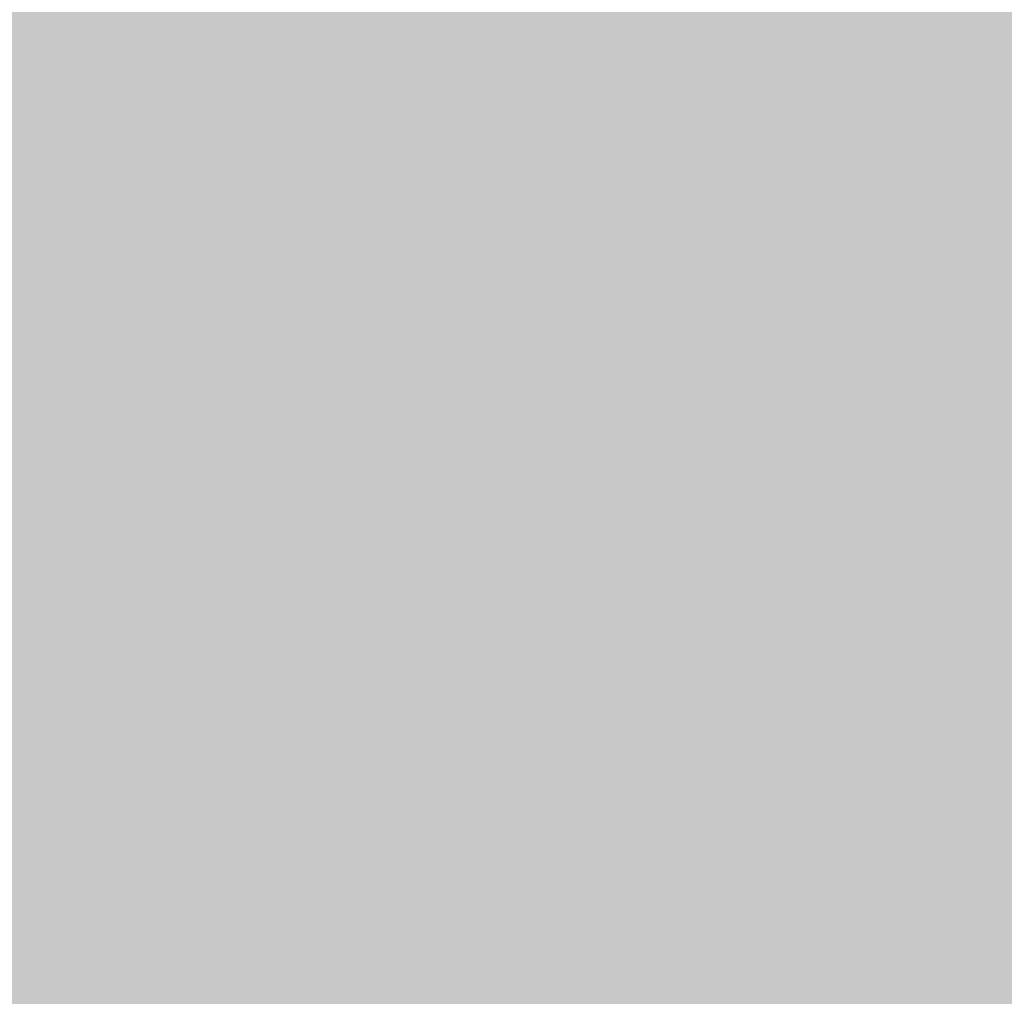
# Model space of a CAD drawing. Units: inches. Extents: x 2083 to 3317, y 1141 to 2115.
# Tile 160 of 256: x 3126.955939 to 3126.958245, y 1263.263648 to 1263.265937. Entities that reach past the tile are written whole.
import ezdxf

# ---------------------------------------------------------------- set-up
doc = ezdxf.new("R2010")
doc.units = ezdxf.units.IN
doc.layers.add('A-WALL-PATT', color=251, linetype='Continuous', lineweight=13, true_color=0x636466)

msp = doc.modelspace()

# ---------------------------------------------------------------- hatches: boundary and pattern name
at = {"layer": 'A-WALL-PATT'}
h = msp.add_hatch(color=256, dxfattribs=at)
h.dxf.hatch_style = 1
h.paths.add_polyline_path([(3126.9597832, 2020.7613601), (2748.9597832, 2020.7613601), (2604.9597832, 2020.7613601), (2226.9597832, 2020.7613601), (2226.9597832, 1702.7613601), (2466.9597832, 1702.7613601), (2466.9597832, 1582.7613601), (2418.9597832, 1582.7613601), (2418.9597832, 1477.7613601), (2226.9597832, 1477.7613601), (2226.9597832, 1263.2613601), (2544.9597832, 1263.2613601), (2544.9597832, 1411.7613601), (2604.9597832, 1411.7613601), (2685.9597832, 1411.7613601), (2685.9597832, 1420.7613601), (2604.9597832, 1420.7613601), (2604.9597832, 1573.7613601), (2604.9597832, 1702.7613601), (2604.9597832, 2011.7613601), (2748.9597832, 2011.7613601), (2748.9597832, 1702.7613601), (2862.9597832, 1702.7613601), (2862.9597832, 1621.7613601), (2871.9597832, 1621.7613601), (2871.9597832, 1702.7613601), (2883.9597832, 1702.7613601), (2883.9597832, 1706.9394595, -0.026459), (2883.9597832, 1711.7613601), (2757.9597832, 1711.7613601), (2757.9597832, 1807.7613601), (2787.9597832, 1807.7613601), (2787.9597832, 1812.2613601), (2757.9597832, 1812.2613601), (2757.9597832, 2011.7613601), (2877.9597832, 2011.7613601), (2877.9597832, 1812.2613601), (2847.9597832, 1812.2613601), (2847.9597832, 1807.7613601), (2889.8357425, 1807.7613601), (2889.8357425, 1812.2613601), (2882.4597832, 1812.2613601), (2882.4597832, 2011.7613601), (3117.9597832, 2011.7613601), (3117.9597832, 1812.2613601), (2937.8357425, 1812.2613601), (2937.8357425, 1807.7613601), (2995.7097832, 1807.7613601), (2995.7097832, 1796.1176655), (3000.2097832, 1796.1176655), (3000.2097832, 1807.7613601), (3117.9597832, 1807.7613601), (3117.9597832, 1711.7613601), (3000.2097832, 1711.7613601), (3000.2097832, 1760.1176655), (2998.5727047, 1760.1176655, -0.020711), (2995.7097832, 1760.1176655), (2995.7097832, 1711.7613601), (2931.9597832, 1711.7613601), (2931.9597832, 1702.7613601), (3126.9597832, 1702.7613601)])
h.paths.add_polyline_path([(2471.4597832, 2011.7613601), (2471.4597832, 1810.0113601), (2462.7169357, 1810.0113601), (2462.7169357, 1805.5113601), (2505.9597832, 1805.5113601), (2505.9597832, 1810.0113601), (2475.9597832, 1810.0113601), (2475.9597832, 2011.7613601), (2595.9597832, 2011.7613601), (2595.9597832, 1810.0113601), (2565.9597832, 1810.0113601), (2565.9597832, 1805.5113601), (2595.9597832, 1805.5113601), (2595.9597832, 1711.7613601), (2235.9597832, 1711.7613601), (2235.9597832, 1805.5113601), (2353.7097832, 1805.5113601), (2353.7097832, 1796.0541624), (2358.2097832, 1796.0541624), (2358.2097832, 1805.5113601), (2414.7169357, 1805.5113601), (2414.7169357, 1810.0113601), (2235.9597832, 1810.0113601), (2235.9597832, 2011.7613601)], flags=16)
h.paths.add_polyline_path([(2270.2047343, 1994.6100082), (2270.2047343, 1970.6100082), (2246.2047343, 1970.6100082), (2246.2047343, 1994.6100082)], flags=0)
edge = h.paths.add_edge_path(flags=0)
edge.add_ellipse((2332.027391, 1899.7981761), major_axis=(-3.0429938, 3.0429938), ratio=0.16825245, start_angle=-161.3321656, end_angle=-156.3071136, ccw=False)
edge.add_ellipse((2333.0820373, 1898.7435297), major_axis=(-1.0546463, 1.0546463), ratio=0.453532097, start_angle=-123.371019, end_angle=-94.1591066)
edge = h.paths.add_edge_path(flags=0)
edge.add_ellipse((2332.027391, 1968.8762897), major_axis=(3.0429938, 3.0429938), ratio=0.16825245, start_angle=18.6678344, end_angle=23.6928864)
edge.add_spline(control_points=[(2332.9255964, 1970.6911045), (2332.2267681, 1970.3360997), (2330.8937087, 1969.6589054), (2328.4130803, 1970.9321376), (2327.2039345, 1967.7487119), (2324.7095965, 1969.9555886), (2322.5328223, 1967.012354), (2320.0128462, 1971.2958124), (2317.6803077, 1968.1578449), (2316.0405263, 1967.1020468), (2315.4269045, 1966.8096022)], knot_values=[0, 0, 0, 0, 2.267059, 4.324559, 6.685584, 8.878641, 11.121502, 14.300359, 17.755284, 19.732645, 19.732645, 19.732645, 19.732645], degree=3, periodic=0)
edge.add_ellipse((2332.027391, 1968.8762897), major_axis=(3.0429938, 3.0429938), ratio=0.16825245, start_angle=18.6678344, end_angle=23.6928864, ccw=False)
edge.add_ellipse((2333.0820373, 1969.930936), major_axis=(1.0546463, 1.0546463), ratio=0.453532097, start_angle=56.628981, end_angle=85.8408934, ccw=False)
edge = h.paths.add_edge_path(flags=0)
edge.add_spline(control_points=[(2296.4282874, 1967.9879081), (2293.6278045, 1965.3363137), (2287.7036238, 1959.727094), (2299.7438601, 1949.9956993), (2294.5325909, 1935.6685275), (2290.5732281, 1920.6035119), (2293.3941244, 1909.9736911), (2296.1854073, 1904.9665431)], knot_values=[0.099185, 0.099185, 0.099185, 0.099185, 0.345301, 0.619822, 0.982653, 1.386093, 1.810555, 1.810555, 1.810555, 1.810555], degree=3, periodic=0)
edge.add_spline(control_points=[(2296.1854073, 1904.9665431), (2297.3835817, 1902.6193002), (2298.0009694, 1901.9493116), (2298.5529698, 1901.4681549)], knot_values=[0.006246, 0.006246, 0.006246, 0.006246, 0.055476, 0.055476, 0.055476, 0.055476], degree=3, periodic=0)
edge.add_spline(control_points=[(2298.5529698, 1901.4681549), (2297.2586121, 1900.9232238), (2295.2252939, 1900.2321257), (2293.0602287, 1900.6142053), (2292.1014227, 1900.788415), (2292.0895776, 1900.790568)], knot_values=[0.312835, 0.312835, 0.312835, 0.312835, 0.40178, 0.474987, 0.475903, 0.475903, 0.475903, 0.475903], degree=3, periodic=0)
edge.add_arc((2292.7936464, 1904.6641088), 3.9370079, 215.4208969, 259.6981795, ccw=False)
edge.add_spline(control_points=[(2289.5853139, 1902.3823039), (2289.4766524, 1902.5350874), (2289.3684805, 1902.6880353), (2289.2608648, 1902.8411699)], knot_values=[0.102872, 0.102872, 0.102872, 0.102872, 0.116896, 0.116896, 0.116896, 0.116896], degree=3, periodic=0)
edge.add_spline(control_points=[(2289.2608648, 1902.8411699), (2288.6866042, 1902.5501922), (2287.6400477, 1902.0199025), (2285.8813368, 1901.8739536), (2283.8529717, 1901.5043521), (2281.7199871, 1899.7105375), (2278.4669913, 1899.492942), (2276.1571361, 1901.8832022), (2272.2589526, 1899.8040711), (2267.7776054, 1901.8431828), (2262.2438819, 1900.1840326), (2257.414927, 1901.7820606), (2254.318374, 1900.7261196), (2253.1782849, 1900.3373431)], knot_values=[0, 0, 0, 0, 1.907977, 3.477176, 5.261074, 7.972851, 11.680248, 13.717921, 16.939592, 22.789562, 27.502503, 33.595215, 37.145618, 37.145618, 37.145618, 37.145618], degree=3, periodic=0)
edge.add_line((2253.1782849, 1900.3373431), (2250.2442397, 1902.8411699))
edge.add_line((2250.2442397, 1902.8411699), (2250.2442397, 1965.8332959))
edge.add_line((2250.2442397, 1965.8332959), (2253.1782849, 1968.3371226))
edge.add_spline(control_points=[(2253.1782849, 1968.3371226), (2254.318374, 1967.9483462), (2257.414927, 1966.8924051), (2262.2438819, 1968.4904332), (2267.7776054, 1966.8312829), (2271.5267301, 1968.5372172), (2273.8759143, 1967.8282895), (2274.2067012, 1967.7276424)], knot_values=[0, 0, 0, 0, 0.09018, 0.244935, 0.364644, 0.513233, 0.537855, 0.537855, 0.537855, 0.537855], degree=3, periodic=0)
edge.add_arc((2274.3528869, 1963.7933495), 3.9370079, 72.0511336, 92.1279492, ccw=False)
edge.add_arc((2281.2969331, 1985.2300027), 18.5962982, 252.05113361, 288.56572166)
edge.add_arc((2292.3167172, 1956.0288805), 12.6460805, 71.02678788, 113.77821843, ccw=False)
edge = h.paths.add_edge_path(flags=0)
edge.add_spline(control_points=[(2274.8994147, 1951.8561946), (2275.066156, 1951.6165924), (2275.2326866, 1951.3765878), (2275.3979871, 1951.1358545)], knot_values=[1.409916, 1.409916, 1.409916, 1.409916, 1.43159, 1.43159, 1.43159, 1.43159], degree=3, periodic=0)
edge.add_spline(control_points=[(2275.3979871, 1951.1358545), (2275.7921055, 1950.5618854), (2276.1792311, 1949.9837745), (2276.5455462, 1949.3971029)], knot_values=[1.358238, 1.358238, 1.358238, 1.358238, 1.409916, 1.409916, 1.409916, 1.409916], degree=3, periodic=0)
edge.add_line((2276.5455462, 1949.3971029), (2277.437289, 1947.8621847))
edge.add_spline(control_points=[(2277.437289, 1947.8621847), (2276.3038341, 1945.6731147), (2274.6396979, 1942.4268817), (2274.631615, 1938.0938998), (2272.7991237, 1930.8515498), (2274.3564261, 1943.8970461), (2275.9476814, 1947.9233558), (2276.5455462, 1949.3971029)], knot_values=[0.005632, 0.005632, 0.005632, 0.005632, 0.186014, 0.266002, 0.357087, 0.59639, 0.739732, 0.739732, 0.739732, 0.739732], degree=3, periodic=0)
edge.add_spline(control_points=[(2276.5455462, 1949.3971029), (2276.1792311, 1949.9837745), (2275.7921055, 1950.5618854), (2275.3979871, 1951.1358545)], knot_values=[1.358238, 1.358238, 1.358238, 1.358238, 1.409916, 1.409916, 1.409916, 1.409916], degree=3, periodic=0)
edge.add_spline(control_points=[(2275.3979871, 1951.1358545), (2274.9425002, 1950.0804523), (2274.2077604, 1948.0252718), (2273.9346018, 1944.8514774), (2272.4685341, 1937.6274891), (2273.4662155, 1945.6964663), (2274.7006154, 1951.0594725), (2274.8994147, 1951.8561946)], knot_values=[0.104364, 0.104364, 0.104364, 0.104364, 0.189636, 0.269624, 0.36071, 0.600013, 0.644622, 0.644622, 0.644622, 0.644622], degree=3, periodic=0)
h.paths.add_polyline_path([(2269.1675139, 1963.1275729, -0.357527), (2268.170633, 1960.9763695, -0.092561), (2268.170633, 1939.4363249, -0.357527), (2269.1675139, 1937.2851215, -0.357527), (2267.0163105, 1938.2820024, -0.164785), (2254.6855813, 1938.2820024, -0.357527), (2252.5343779, 1937.2851215, -0.357527), (2253.5312587, 1939.4363249, -0.092561), (2253.5312587, 1960.9763695, -0.357527), (2252.5343779, 1963.1275729, -0.357527), (2254.6855813, 1962.130692, -0.164785), (2267.0163105, 1962.130692, -0.357527)], flags=0)
h.paths.add_polyline_path([(2248.8740679, 1967.8017998), (2248.8740679, 1957.0277095), (2249.4577833, 1957.0277095), (2249.4577833, 1911.6467562), (2248.8740679, 1911.6467562), (2248.8740679, 1900.8726659), (2246.5118632, 1900.8726659, 0.197327), (2244.1496584, 1902.4568734), (2244.1496584, 1966.2175923, 0.197327), (2246.5118632, 1967.8017998)], flags=0)
h.paths.add_polyline_path([(2269.1675139, 1931.3893442, -0.357527), (2268.170633, 1929.2381408, -0.092561), (2268.170633, 1907.6980962, -0.357527), (2269.1675139, 1905.5468928, -0.357527), (2267.0163105, 1906.5437737, -0.164785), (2254.6855813, 1906.5437737, -0.357527), (2252.5343779, 1905.5468928, -0.357527), (2253.5312587, 1907.6980962, -0.092561), (2253.5312587, 1929.2381408, -0.357527), (2252.5343779, 1931.3893442, -0.357527), (2254.6855813, 1930.3924634, -0.164785), (2267.0163105, 1930.3924634, -0.357527)], flags=0)
edge = h.paths.add_edge_path(flags=0)
edge.add_spline(control_points=[(2276.1968578, 1906.7237016), (2276.1681442, 1909.0289278), (2276.1140492, 1913.371852), (2270.5984171, 1924.9249783), (2273.9051746, 1919.0127787), (2275.9217115, 1916.2620626), (2275.4745699, 1912.4021495), (2277.2578735, 1910.3806206), (2276.6960436, 1908.2250358), (2276.6462176, 1906.8130226), (2276.6178249, 1906.0084068)], knot_values=[0, 0, 0, 0, 8.61026, 16.221274, 18.843057, 23.804898, 27.440828, 29.356102, 31.203478, 33.650687, 33.650687, 33.650687, 33.650687], degree=3, periodic=0)
edge.add_spline(control_points=[(2276.6178249, 1906.0084068), (2276.6233131, 1905.6241436), (2276.4977381, 1904.6286608), (2275.4417789, 1903.8547251), (2274.9373144, 1903.0804497), (2274.8590804, 1902.8411699)], knot_values=[0.156488, 0.156488, 0.156488, 0.156488, 0.184398, 0.231376, 0.250598, 0.250598, 0.250598, 0.250598], degree=3, periodic=0)
edge.add_line((2274.8590804, 1902.8411699), (2276.50598, 1902.8411699))
edge.add_spline(control_points=[(2276.50598, 1902.8411699), (2276.7883084, 1903.0849395), (2277.6650711, 1904.1251958), (2278.2495378, 1904.340738), (2277.6538719, 1908.5273866), (2278.15567, 1906.2278078), (2278.100464, 1905.2859484), (2278.8466748, 1904.0690054), (2277.8567853, 1903.4149482), (2277.8741909, 1902.9910497), (2277.9035616, 1902.8411699)], knot_values=[0.059574, 0.059574, 0.059574, 0.059574, 0.080753, 0.103741, 0.16972, 0.176036, 0.207137, 0.240474, 0.262341, 0.27366, 0.27366, 0.27366, 0.27366], degree=3, periodic=0)
edge.add_line((2277.9035616, 1902.8411699), (2280.0298255, 1902.8411699))
edge.add_spline(control_points=[(2280.0298255, 1902.8411699), (2279.8882214, 1903.088398), (2279.4992571, 1903.9815512), (2280.1522839, 1905.9393491), (2278.103615, 1909.6577572), (2279.7623946, 1907.185285), (2280.3279002, 1904.8748608), (2280.4851086, 1903.4895904), (2281.4632687, 1903.2494323), (2281.7583431, 1902.9364967), (2281.8340361, 1902.8411699)], knot_values=[0.013856, 0.013856, 0.013856, 0.013856, 0.034874, 0.088867, 0.107879, 0.126738, 0.158714, 0.193757, 0.217487, 0.226722, 0.226722, 0.226722, 0.226722], degree=3, periodic=0)
edge.add_spline(control_points=[(2281.8340361, 1902.8411699), (2281.7875348, 1902.8267029), (2281.6470224, 1902.7829881), (2281.3955272, 1902.85949), (2281.088077, 1902.9852418), (2280.7206826, 1903.060902), (2280.3334513, 1903.0257257), (2280.1247668, 1902.898879), (2280.0298255, 1902.8411699)], knot_values=[0, 0, 0, 0, 0.14413, 0.435517, 0.749276, 1.153046, 1.548371, 1.878348, 1.878348, 1.878348, 1.878348], degree=3, periodic=0)
edge.add_line((2280.0298255, 1902.8411699), (2277.9035616, 1902.8411699))
edge.add_spline(control_points=[(2277.9035616, 1902.8411699), (2277.892855, 1902.7958553), (2277.865396, 1902.6796374), (2277.6074793, 1902.6874828), (2277.2740503, 1902.8006999), (2276.8379209, 1902.6197745), (2276.5838074, 1902.7892611), (2276.50598, 1902.8411699)], knot_values=[0, 0, 0, 0, 0.127189, 0.326199, 0.628009, 1.24357, 1.515331, 1.515331, 1.515331, 1.515331], degree=3, periodic=0)
edge.add_line((2276.50598, 1902.8411699), (2274.8590804, 1902.8411699))
edge.add_spline(control_points=[(2274.8590804, 1902.8411699), (2274.8144367, 1902.8985868), (2274.7251297, 1903.013446), (2274.4934765, 1903.1189684), (2274.2442854, 1902.9605386), (2273.9371207, 1903.1849416), (2273.6140395, 1902.9831428), (2273.4083164, 1902.8830449), (2273.322254, 1902.8411699)], knot_values=[0, 0, 0, 0, 0.21843, 0.436957, 0.687977, 0.990379, 1.398396, 1.69185, 1.69185, 1.69185, 1.69185], degree=3, periodic=0)
edge.add_spline(control_points=[(2273.322254, 1902.8411699), (2273.6167403, 1903.445692), (2274.2739977, 1904.5382529), (2276.0272387, 1904.5737017), (2276.2069634, 1906.5836372), (2276.1968578, 1906.7237016)], knot_values=[0.012227, 0.012227, 0.012227, 0.012227, 0.059472, 0.106218, 0.134458, 0.134458, 0.134458, 0.134458], degree=3, periodic=0)
h.paths.add_polyline_path([(2270.7760538, 1897.7898284), (2270.7760538, 1873.7898284), (2246.7760538, 1873.7898284), (2246.7760538, 1897.7898284)], flags=0)
h.paths.add_polyline_path([(2353.7097832, 1760.0050593), (2353.7097832, 1760.0541624), (2358.2097832, 1760.0541624, -0.033729)], flags=0)
h.paths.add_polyline_path([(2321.8191188, 1737.5291862), (2341.9953271, 1737.5291862, -0.414214), (2343.2032727, 1736.3212406), (2343.2032727, 1721.0205964, -0.414214), (2341.9953271, 1719.8126508), (2321.8191188, 1719.8126508, -0.414214), (2320.6111732, 1721.0205964), (2320.6111732, 1736.3212406, -0.414214)], flags=0)
h.paths.add_polyline_path([(2324.2350099, 1736.3212406), (2339.5794359, 1736.3212406, -0.414214), (2341.9953271, 1733.9053494), (2341.9953271, 1725.4497302, -0.414214), (2339.5794359, 1723.033839), (2333.6805885, 1723.033839), (2333.8453172, 1722.0454666, -0.870646), (2335.4253988, 1721.8258934, -0.767327), (2333.922694, 1721.4232449), (2331.2910241, 1721.4232449, -0.767327), (2329.7883193, 1721.8258934, -0.870646), (2331.3684009, 1722.0454666), (2331.5331296, 1723.033839), (2324.2350099, 1723.033839, -0.414214), (2321.8191188, 1725.4497302), (2321.8191188, 1733.9053494, -0.414214)], flags=0)
h.paths.add_polyline_path([(2570.4837892, 1928.6154443), (2589.6837892, 1928.6154443), (2590.1688286, 1928.6154443), (2590.1688286, 1904.9933971), (2570.4837892, 1904.9933971)], flags=0)
h.paths.add_polyline_path([(2574.4473242, 1927.2638215, -1), (2572.8288357, 1927.2638215, -1)], flags=0)
h.paths.add_polyline_path([(2573.0898665, 1926.9408768), (2573.925032, 1927.7760423), (2574.1477428, 1927.5533315), (2573.3125773, 1926.718166)], flags=0)
h.paths.add_polyline_path([(2578.7790648, 1919.7296175, -1), (2571.5916632, 1919.7296175, -1)], flags=0)
h.paths.add_polyline_path([(2578.385364, 1919.7296175, -1), (2571.985364, 1919.7296175, -1)], flags=0)
h.paths.add_polyline_path([(2331.5957638, 1729.4762156, -1), (2333.6179542, 1729.4762156, -1)], flags=0)
h.paths.add_polyline_path([(2578.0342282, 1927.2638215, -1), (2576.4157396, 1927.2638215, -1)], flags=0)
h.paths.add_polyline_path([(2576.6888513, 1927.5310886), (2576.9115621, 1927.7537993), (2577.7467276, 1926.9186339), (2577.5240168, 1926.6959231)], flags=0)
h.paths.add_polyline_path([(2578.1390648, 1909.8595388, -1), (2572.2316632, 1909.8595388, -1)], flags=0)
h.paths.add_polyline_path([(2577.745364, 1909.8595388, -1), (2572.625364, 1909.8595388, -1)], flags=0)
h.paths.add_polyline_path([(2583.7977179, 1927.2638215, -1), (2582.1792294, 1927.2638215, -1)], flags=0)
h.paths.add_polyline_path([(2582.7186487, 1927.7537993), (2583.5538142, 1926.9186339), (2583.3311034, 1926.6959231), (2582.4959379, 1927.5310886)], flags=0)
h.paths.add_polyline_path([(2582.4959379, 1927.5310886), (2582.7186487, 1927.7537993), (2583.5538142, 1926.9186339), (2583.3311034, 1926.6959231)], flags=0)
h.paths.add_polyline_path([(2587.7390648, 1920.5296175, -1), (2581.8316632, 1920.5296175, -1)], flags=0)
h.paths.add_polyline_path([(2587.345364, 1920.5296175, -1), (2582.225364, 1920.5296175, -1)], flags=0)
h.paths.add_polyline_path([(2587.3846219, 1927.2638215, -1), (2585.7661333, 1927.2638215, -1)], flags=0)
h.paths.add_polyline_path([(2586.0819925, 1926.9802469), (2586.917158, 1927.8154124), (2587.1398688, 1927.5927016), (2586.3047033, 1926.7575361)], flags=0)
h.paths.add_polyline_path([(2588.3790648, 1910.6595388, -1), (2581.1916632, 1910.6595388, -1)], flags=0)
h.paths.add_polyline_path([(2587.985364, 1910.6595388, -1), (2581.585364, 1910.6595388, -1)], flags=0)
h.paths.add_polyline_path([(2417.1677288, 1729.4778955), (2437.3439372, 1729.4778955, -0.414214), (2438.5518828, 1728.2699499), (2438.5518828, 1712.9693057, -0.414214), (2437.3439372, 1711.7613601), (2417.1677288, 1711.7613601, -0.414214), (2415.9597832, 1712.9693057), (2415.9597832, 1728.2699499, -0.414214)], flags=0)
h.paths.add_polyline_path([(2419.58362, 1728.2699499), (2434.928046, 1728.2699499, -0.414214), (2437.3439372, 1725.8540587), (2437.3439372, 1717.3984395, -0.414214), (2434.928046, 1714.9825483), (2429.0291985, 1714.9825483), (2429.1939273, 1713.9941758, -0.870646), (2430.7740089, 1713.7746027, -0.767327), (2429.2713041, 1713.3719542), (2426.6396342, 1713.3719542, -0.767327), (2425.1369294, 1713.7746027, -0.870646), (2426.717011, 1713.9941758), (2426.8817397, 1714.9825483), (2419.58362, 1714.9825483, -0.414214), (2417.1677288, 1717.3984395), (2417.1677288, 1725.8540587, -0.414214)], flags=0)
h.paths.add_polyline_path([(2419.58362, 1728.2699499), (2434.928046, 1728.2699499, -0.414214), (2437.3439372, 1725.8540587), (2437.3439372, 1717.3984395, -0.414214), (2434.928046, 1714.9825483), (2429.0291985, 1714.9825483), (2428.3581177, 1719.0090337), (2427.5528206, 1719.0090337), (2426.8817397, 1714.9825483), (2419.58362, 1714.9825483, -0.414214), (2417.1677288, 1717.3984395), (2417.1677288, 1725.8540587, -0.414214)], flags=0)
h.paths.add_polyline_path([(2426.9443739, 1721.4249248, -1), (2428.9665643, 1721.4249248, -1)], flags=0)
h.paths.add_polyline_path([(2475.9597832, 1702.7613601), (2595.9597832, 1702.7613601), (2595.9597832, 1582.7613601), (2475.9597832, 1582.7613601)], flags=16)
h.paths.add_polyline_path([(2427.9597832, 1573.7613601), (2595.9597832, 1573.7613601), (2595.9597832, 1468.7613601), (2595.9597832, 1420.7613601), (2384.4597832, 1420.7613601), (2384.4597832, 1468.7613601), (2427.9597832, 1468.7613601)], flags=16)
h.paths.add_polyline_path([(2379.9597832, 1468.7613601), (2379.9597832, 1420.7613601), (2235.9597832, 1420.7613601), (2235.9597832, 1468.7613601)], flags=16)
h.paths.add_polyline_path([(2317.8159962, 1466.695767), (2337.9922045, 1466.695767, -0.414214), (2339.2001501, 1465.4878214), (2339.2001501, 1450.1871771, -0.414214), (2337.9922045, 1448.9792315), (2317.8159962, 1448.9792315, -0.414214), (2316.6080506, 1450.1871771), (2316.6080506, 1465.4878214, -0.414214)], flags=0)
h.paths.add_polyline_path([(2320.2318874, 1465.4878214), (2335.5763133, 1465.4878214, -0.414214), (2337.9922045, 1463.0719302), (2337.9922045, 1454.616311, -0.414214), (2335.5763133, 1452.2004198), (2329.6774659, 1452.2004198), (2329.8421946, 1451.2120473, -0.870646), (2331.4222762, 1450.9924742, -0.767327), (2329.9195714, 1450.5898257), (2327.2879015, 1450.5898257, -0.767327), (2325.7851967, 1450.9924742, -0.870646), (2327.3652783, 1451.2120473), (2327.530007, 1452.2004198), (2320.2318874, 1452.2004198, -0.414214), (2317.8159962, 1454.616311), (2317.8159962, 1463.0719302, -0.414214)], flags=0)
h.paths.add_polyline_path([(2320.2318874, 1465.4878214), (2335.5763133, 1465.4878214, -0.414214), (2337.9922045, 1463.0719302), (2337.9922045, 1454.616311, -0.414214), (2335.5763133, 1452.2004198), (2329.6774659, 1452.2004198), (2329.006385, 1456.2269051), (2328.2010879, 1456.2269051), (2327.530007, 1452.2004198), (2320.2318874, 1452.2004198, -0.414214), (2317.8159962, 1454.616311), (2317.8159962, 1463.0719302, -0.414214)], flags=0)
h.paths.add_polyline_path([(2327.5926413, 1458.6427963, -1), (2329.6148317, 1458.6427963, -1)], flags=0)
h.paths.add_polyline_path([(2244.4117436, 1433.3404531), (2241.9209449, 1433.3404531, -0.414214), (2240.0178562, 1435.2435418), (2240.0178562, 1440.9528078, -0.414211), (2241.920925, 1442.8558965), (2244.4117436, 1442.8558965, -1.976472)], flags=0)
h.paths.add_polyline_path([(2245.3568884, 1434.3975358, -0.414214), (2245.3568884, 1441.7988138, -2.144098)], flags=0)
h.paths.add_polyline_path([(2535.9597832, 1416.2613601), (2535.9597832, 1272.2613601), (2235.9597832, 1272.2613601), (2235.9597832, 1416.2613601)], flags=16)
h.paths.add_polyline_path([(2260.1195614, 1384.2928413), (2260.1195614, 1362.0386487), (2237.8653688, 1362.0386487), (2237.8653688, 1384.2928413)], flags=0)
edge = h.paths.add_edge_path(flags=0)
edge.add_line((2318.2518466, 1362.0932983), (2318.1457968, 1362.0009726))
edge.add_ellipse((2317.4451158, 1360.4310442), major_axis=(2.8216404, 2.8216404), ratio=0.16825245, start_angle=18.6678344, end_angle=20.9481273, ccw=False)
edge.add_ellipse((2318.4230451, 1361.4089735), major_axis=(0.9779293, 0.9779293), ratio=0.453532097, start_angle=56.628981, end_angle=70.2262012, ccw=False)
edge = h.paths.add_edge_path(flags=0)
edge.add_line((2319.1073699, 1295.5710784), (2319.0150442, 1295.6771282))
edge.add_ellipse((2317.4451158, 1296.3778091), major_axis=(-2.8216404, 2.8216404), ratio=0.16825245, start_angle=-161.3321656, end_angle=-159.0518727, ccw=False)
edge.add_ellipse((2318.4230451, 1295.3998798), major_axis=(-0.9779293, 0.9779293), ratio=0.453532097, start_angle=-123.371019, end_angle=-109.7737988)
edge = h.paths.add_edge_path(flags=0)
edge.add_spline(control_points=[(2284.2103489, 1301.1702189), (2284.5806878, 1300.444719), (2284.8911891, 1299.8920243), (2285.159553, 1299.4610182)], knot_values=[0.039066, 0.039066, 0.039066, 0.039066, 0.055476, 0.055476, 0.055476, 0.055476], degree=3, periodic=0)
edge.add_line((2285.159553, 1299.4610182), (2284.2103489, 1301.1702189))
edge = h.paths.add_edge_path(flags=0)
edge.add_line((2280.4124579, 1297.2980125), (2283.3699905, 1297.0361216))
edge.add_line((2283.3699905, 1297.0361216), (2286.4056902, 1297.9263104))
edge.add_spline(control_points=[(2286.4056902, 1297.9263104), (2285.305487, 1297.4631193), (2284.3447774, 1297.1291508), (2283.3699905, 1297.0361216)], knot_values=[0.394369, 0.394369, 0.394369, 0.394369, 0.475903, 0.475903, 0.475903, 0.475903], degree=3, periodic=0)
edge.add_spline(control_points=[(2283.3699905, 1297.0361216), (2283.2813895, 1297.027666), (2282.316289, 1296.9573356), (2281.3125019, 1297.1344787), (2280.4234414, 1297.2960161), (2280.4124579, 1297.2980125)], knot_values=[0.312835, 0.312835, 0.312835, 0.312835, 0.320246, 0.393453, 0.394369, 0.394369, 0.394369, 0.394369], degree=3, periodic=0)
edge = h.paths.add_edge_path(flags=0)
edge.add_line((2284.4355615, 1359.6072854), (2280.4462909, 1355.328047))
edge.add_line((2280.4462909, 1355.328047), (2279.5799868, 1351.0177544))
edge.add_line((2279.5799868, 1351.0177544), (2282.4129737, 1346.5804327))
edge.add_spline(control_points=[(2282.4129737, 1346.5804327), (2283.1533308, 1345.5892358), (2284.2528957, 1344.0288973), (2284.801037, 1342.3871671), (2284.9351625, 1341.8055443)], knot_values=[1.240098, 1.240098, 1.240098, 1.240098, 1.332892, 1.382712, 1.382712, 1.382712, 1.382712], degree=3, periodic=0)
edge.add_spline(control_points=[(2284.9351625, 1341.8055443), (2285.3191079, 1340.1406002), (2285.2330291, 1338.4092041), (2284.9099384, 1336.6541222)], knot_values=[1.097484, 1.097484, 1.097484, 1.097484, 1.240098, 1.240098, 1.240098, 1.240098], degree=3, periodic=0)
edge.add_spline(control_points=[(2284.9099384, 1336.6541222), (2284.5868478, 1334.8990403), (2284.0267453, 1333.1202725), (2283.4626437, 1331.3605849)], knot_values=[0.95487, 0.95487, 0.95487, 0.95487, 1.097484, 1.097484, 1.097484, 1.097484], degree=3, periodic=0)
edge.add_line((2283.4626437, 1331.3605849), (2281.8903759, 1326.153357))
edge.add_line((2281.8903759, 1326.153357), (2280.7562592, 1321.0560888))
edge.add_line((2280.7562592, 1321.0560888), (2280.2992048, 1316.0019772))
edge.add_line((2280.2992048, 1316.0019772), (2280.7159327, 1310.9500678))
edge.add_line((2280.7159327, 1310.9500678), (2282.0280939, 1305.9721367))
edge.add_line((2282.0280939, 1305.9721367), (2284.2103489, 1301.1702189))
edge.add_spline(control_points=[(2284.2103489, 1301.1702189), (2283.3407305, 1302.7301854), (2282.6119044, 1304.3364933), (2282.0280939, 1305.9721367)], knot_values=[0.099185, 0.099185, 0.099185, 0.099185, 0.241799, 0.241799, 0.241799, 0.241799], degree=3, periodic=0)
edge.add_spline(control_points=[(2282.0280939, 1305.9721367), (2281.4442835, 1307.6077801), (2281.0054886, 1309.2727591), (2280.7159327, 1310.9500678)], knot_values=[0.241799, 0.241799, 0.241799, 0.241799, 0.384413, 0.384413, 0.384413, 0.384413], degree=3, periodic=0)
edge.add_spline(control_points=[(2280.7159327, 1310.9500678), (2280.4332411, 1312.5876134), (2280.2893863, 1314.2769594), (2280.2988938, 1315.9620324), (2280.2992048, 1316.0019772)], knot_values=[0.384413, 0.384413, 0.384413, 0.384413, 0.523647, 0.527028, 0.527028, 0.527028, 0.527028], degree=3, periodic=0)
edge.add_spline(control_points=[(2280.2992048, 1316.0019772), (2280.3123257, 1317.6869552), (2280.4778706, 1319.3679256), (2280.7562592, 1321.0560888)], knot_values=[0.527028, 0.527028, 0.527028, 0.527028, 0.669642, 0.669642, 0.669642, 0.669642], degree=3, periodic=0)
edge.add_spline(control_points=[(2280.7562592, 1321.0560888), (2281.0346478, 1322.7442519), (2281.4258801, 1324.4396079), (2281.8903759, 1326.153357)], knot_values=[0.669642, 0.669642, 0.669642, 0.669642, 0.812256, 0.812256, 0.812256, 0.812256], degree=3, periodic=0)
edge.add_spline(control_points=[(2281.8903759, 1326.153357), (2282.2643834, 1327.5332507), (2282.7878702, 1329.2618097), (2283.352751, 1331.0177803), (2283.4626437, 1331.3605849)], knot_values=[0.812256, 0.812256, 0.812256, 0.812256, 0.927087, 0.95487, 0.95487, 0.95487, 0.95487], degree=3, periodic=0)
edge.add_line((2283.4626437, 1331.3605849), (2284.9099384, 1336.6541222))
edge.add_line((2284.9099384, 1336.6541222), (2284.9351625, 1341.8055443))
edge.add_line((2284.9351625, 1341.8055443), (2282.4129737, 1346.5804327))
edge.add_spline(control_points=[(2282.4129737, 1346.5804327), (2281.2751273, 1348.1037918), (2280.0784467, 1349.5703178), (2279.5799868, 1351.0177544)], knot_values=[1.382712, 1.382712, 1.382712, 1.382712, 1.525326, 1.525326, 1.525326, 1.525326], degree=3, periodic=0)
edge.add_spline(control_points=[(2279.5799868, 1351.0177544), (2279.4432818, 1351.4147209), (2279.1363124, 1352.856922), (2279.7351897, 1354.2903851), (2280.4462909, 1355.328047)], knot_values=[1.525326, 1.525326, 1.525326, 1.525326, 1.564439, 1.667941, 1.667941, 1.667941, 1.667941], degree=3, periodic=0)
edge.add_spline(control_points=[(2280.4462909, 1355.328047), (2281.4261132, 1356.7578354), (2282.9308373, 1358.1825604), (2284.4355615, 1359.6072854)], knot_values=[1.667941, 1.667941, 1.667941, 1.667941, 1.810555, 1.810555, 1.810555, 1.810555], degree=3, periodic=0)
edge.add_arc((2280.6230749, 1348.518181), 11.7261796, 71.02678788, 113.77821843)
edge.add_arc((2270.4048917, 1375.5951559), 17.2435667, 252.05113361, 288.56572166, ccw=False)
edge.add_arc((2263.9659692, 1355.7178471), 3.6506221, 72.0511336, 92.1279492)
edge.add_arc((2263.9659692, 1355.7178471), 3.6506221, 92.1279492, 177.98513)
edge.add_spline(control_points=[(2260.3176041, 1355.8461989), (2260.2604169, 1354.2206683), (2260.551278, 1350.1865469), (2262.9993445, 1346.7662507), (2264.4727415, 1344.6490245)], knot_values=[1.43159, 1.43159, 1.43159, 1.43159, 1.564144, 1.770695, 1.770695, 1.770695, 1.770695], degree=3, periodic=0)
edge.add_line((2264.4727415, 1344.6490245), (2264.9355904, 1343.9825301))
edge.add_spline(control_points=[(2263.8010444, 1340.2481052), (2263.8432379, 1340.5140884), (2264.0672444, 1341.7564652), (2264.5126928, 1343.0024532), (2264.9350468, 1343.9810834)], knot_values=[0.53657, 0.53657, 0.53657, 0.53657, 0.559349, 0.644622, 0.644622, 0.644622, 0.644622], degree=3, periodic=0)
edge.add_spline(control_points=[(2264.9350468, 1343.9810834), (2265.1177715, 1343.7149747), (2265.2988751, 1343.4479058), (2265.4767562, 1343.1793646)], knot_values=[1.384077, 1.384077, 1.384077, 1.384077, 1.409916, 1.409916, 1.409916, 1.409916], degree=3, periodic=0)
edge.add_spline(control_points=[(2265.4767562, 1343.1793646), (2265.6546373, 1342.9108234), (2265.8292958, 1342.64081), (2265.9991301, 1342.368812)], knot_values=[1.358238, 1.358238, 1.358238, 1.358238, 1.384077, 1.384077, 1.384077, 1.384077], degree=3, periodic=0)
edge.add_line((2265.9991301, 1342.368812), (2266.8260057, 1340.9455468))
edge.add_spline(control_points=[(2266.8260057, 1340.9455468), (2268.894401, 1337.0896912), (2271.3981727, 1325.8430009), (2270.5161644, 1310.5685568), (2275.9193759, 1301.860609), (2277.7895113, 1299.1994495)], knot_values=[0.116896, 0.116896, 0.116896, 0.116896, 0.472987, 1.050969, 1.313793, 1.313793, 1.313793, 1.313793], degree=3, periodic=0)
edge.add_spline(control_points=[(2277.7895113, 1299.1994495), (2277.8394051, 1299.1284519), (2277.8894277, 1299.0574975), (2277.9395717, 1298.9865839)], knot_values=[0.109884, 0.109884, 0.109884, 0.109884, 0.116896, 0.116896, 0.116896, 0.116896], degree=3, periodic=0)
edge.add_line((2277.9395717, 1298.9865839), (2277.7888489, 1299.1991139))
edge.add_spline(control_points=[(2277.7888489, 1299.1991139), (2277.2565819, 1298.9294144), (2276.2863504, 1298.4379024), (2275.0393517, 1298.3344186), (2274.3833299, 1298.2388951), (2274.2152543, 1298.209338)], knot_values=[33.12187, 33.12187, 33.12187, 33.12187, 35.029056, 36.598255, 37.144827, 37.144827, 37.144827, 37.144827], degree=3, periodic=0)
edge.add_line((2274.2152543, 1298.209338), (2273.073147, 1297.8929607))
edge.add_spline(control_points=[(2273.073147, 1297.8929607), (2272.3229363, 1297.579784), (2271.0391507, 1296.5105078), (2269.2483948, 1296.2260622), (2268.4231004, 1296.3746543)], knot_values=[26.532584, 26.532584, 26.532584, 26.532584, 29.198919, 31.839101, 31.839101, 31.839101, 31.839101], degree=3, periodic=0)
edge.add_line((2268.4231004, 1296.3746543), (2263.8785014, 1297.4575338))
edge.add_spline(control_points=[(2263.8785014, 1297.4575338), (2263.5560769, 1297.3594345), (2261.8603064, 1296.8386943), (2260.2387805, 1297.2824073), (2258.9334543, 1297.5164611)], knot_values=[15.919551, 15.919551, 15.919551, 15.919551, 16.939592, 21.226067, 21.226067, 21.226067, 21.226067], degree=3, periodic=0)
edge.add_line((2258.9334543, 1297.5164611), (2254.0552332, 1297.3290098))
edge.add_spline(control_points=[(2254.0552332, 1297.3290098), (2253.7555255, 1297.295815), (2252.1136834, 1297.1651738), (2250.4618687, 1297.5442209), (2249.1296862, 1297.6678818)], knot_values=[5.306517, 5.306517, 5.306517, 5.306517, 6.276435, 10.613034, 10.613034, 10.613034, 10.613034], degree=3, periodic=0)
edge.add_line((2249.1296862, 1297.6678818), (2244.3316495, 1296.8777561))
edge.add_line((2244.3316495, 1296.8777561), (2241.6110326, 1299.1994495))
edge.add_line((2241.6110326, 1299.1994495), (2241.6110326, 1357.6094038))
edge.add_line((2241.6110326, 1357.6094038), (2244.3316495, 1359.9310973))
edge.add_line((2244.3316495, 1359.9310973), (2252.7288228, 1359.5426917))
edge.add_spline(control_points=[(2252.7288228, 1359.5426917), (2252.8709387, 1359.5464396), (2253.3057402, 1359.5481716), (2253.7398447, 1359.5142744), (2254.0317419, 1359.4824261)], knot_values=[0.233291, 0.233291, 0.233291, 0.233291, 0.244935, 0.268927, 0.268927, 0.268927, 0.268927], degree=3, periodic=0)
edge.add_line((2254.0317419, 1359.4824261), (2259.5871899, 1359.4163899))
edge.add_spline(control_points=[(2259.5871899, 1359.4163899), (2260.6770676, 1359.6285026), (2262.0731971, 1359.8970025), (2263.5236925, 1359.4592776), (2263.8304173, 1359.3659518)], knot_values=[0.422516, 0.422516, 0.422516, 0.422516, 0.513233, 0.537855, 0.537855, 0.537855, 0.537855], degree=3, periodic=0)
edge.add_arc((2263.9659692, 1355.7178471), 3.6506221, 72.0511336, 92.1279492, ccw=False)
edge.add_arc((2270.4048917, 1375.5951559), 17.2435667, 252.05113361, 288.56572166)
edge.add_arc((2280.6230749, 1348.518181), 11.7261796, 71.02678788, 113.77821843, ccw=False)
h.paths.add_polyline_path([(2240.3405298, 1359.4347149), (2240.3405298, 1349.4443532), (2240.8817846, 1349.4443532), (2240.8817846, 1307.3645001), (2240.3405298, 1307.3645001), (2240.3405298, 1297.3741385), (2238.1501565, 1297.3741385, 0.197327), (2235.9597832, 1298.8431076), (2235.9597832, 1357.9657458, 0.197327), (2238.1501565, 1359.4347149)], flags=0)
h.paths.add_polyline_path([(2259.1577904, 1355.1005005, -0.357527), (2258.2334246, 1353.1057799, -0.092561), (2258.2334246, 1333.1326007, -0.357527), (2259.1577904, 1331.1378801, -0.357527), (2257.1630698, 1332.0622458, -0.164785), (2245.7293022, 1332.0622458, -0.357527), (2243.7345816, 1331.1378801, -0.357527), (2244.6589474, 1333.1326007, -0.092561), (2244.6589474, 1353.1057799, -0.357527), (2243.7345816, 1355.1005005, -0.357527), (2245.7293022, 1354.1761347, -0.164785), (2257.1630698, 1354.1761347, -0.357527)], flags=0)
edge = h.paths.add_edge_path(flags=0)
edge.add_line((2265.9991301, 1342.368812), (2266.8260057, 1340.9455468))
edge.add_line((2266.8260057, 1340.9455468), (2265.3075567, 1337.8140664))
edge.add_line((2265.3075567, 1337.8140664), (2264.358232, 1334.6529388))
edge.add_line((2264.358232, 1334.6529388), (2264.2620123, 1333.7997046))
edge.add_spline(control_points=[(2264.2620123, 1333.7997046), (2264.2083565, 1333.187055), (2264.1620602, 1332.3655252), (2264.0071444, 1331.4139326), (2263.9690487, 1331.2018338)], knot_values=[0.464444, 0.464444, 0.464444, 0.464444, 0.516691, 0.531608, 0.531608, 0.531608, 0.531608], degree=3, periodic=0)
edge.add_spline(control_points=[(2263.9690487, 1331.2018338), (2263.7745349, 1330.1188727), (2263.4243703, 1328.7908386), (2263.2574202, 1328.5306516), (2263.2340282, 1328.5146115)], knot_values=[0.372682, 0.372682, 0.372682, 0.372682, 0.44885, 0.464444, 0.464444, 0.464444, 0.464444], degree=3, periodic=0)
edge.add_spline(control_points=[(2263.2340282, 1328.5146115), (2263.096382, 1328.4202271), (2263.1311696, 1329.3014765), (2263.2749528, 1330.6157493)], knot_values=[0.280919, 0.280919, 0.280919, 0.280919, 0.372682, 0.372682, 0.372682, 0.372682], degree=3, periodic=0)
edge.add_spline(control_points=[(2263.2749528, 1330.6157493), (2263.4187361, 1331.930022), (2263.6715151, 1333.677318), (2263.9698519, 1335.3150268)], knot_values=[0.189157, 0.189157, 0.189157, 0.189157, 0.280919, 0.280919, 0.280919, 0.280919], degree=3, periodic=0)
edge.add_spline(control_points=[(2263.9698519, 1335.3150268), (2264.1004958, 1336.0321917), (2264.4187827, 1337.6219113), (2264.7548476, 1338.8644304), (2264.9474193, 1339.4911244)], knot_values=[0.097394, 0.097394, 0.097394, 0.097394, 0.137578, 0.189157, 0.189157, 0.189157, 0.189157], degree=3, periodic=0)
edge.add_spline(control_points=[(2264.9474193, 1339.4911244), (2265.2900171, 1340.6060546), (2265.6442376, 1341.4939958), (2265.9991301, 1342.368812)], knot_values=[0.005632, 0.005632, 0.005632, 0.005632, 0.097394, 0.097394, 0.097394, 0.097394], degree=3, periodic=0)
h.paths.add_polyline_path([(2259.1577904, 1325.6709733, -0.357527), (2258.2334246, 1323.6762527, -0.092561), (2258.2334246, 1303.7030735, -0.357527), (2259.1577904, 1301.7083529, -0.357527), (2257.1630698, 1302.6327186, -0.164785), (2245.7293022, 1302.6327186, -0.357527), (2243.7345816, 1301.7083529, -0.357527), (2244.6589474, 1303.7030735, -0.092561), (2244.6589474, 1323.6762527, -0.357527), (2243.7345816, 1325.6709733, -0.357527), (2245.7293022, 1324.7466075, -0.164785), (2257.1630698, 1324.7466075, -0.357527)], flags=0)
edge = h.paths.add_edge_path(flags=0)
edge.add_spline(control_points=[(2261.7089377, 1317.3114208), (2261.6794818, 1317.4175798), (2261.7618581, 1317.3885347), (2262.4907358, 1316.0898725), (2262.962185, 1315.3008975)], knot_values=[14.955861, 14.955861, 14.955861, 14.955861, 16.221274, 18.694826, 18.694826, 18.694826, 18.694826], degree=3, periodic=0)
edge.add_spline(control_points=[(2262.962185, 1315.3008975), (2262.9904374, 1315.2536169), (2263.7020958, 1314.0673762), (2264.3489834, 1313.1271533), (2264.7300545, 1312.1641544)], knot_values=[18.694826, 18.694826, 18.694826, 18.694826, 18.843057, 22.433791, 22.433791, 22.433791, 22.433791], degree=3, periodic=0)
edge.add_spline(control_points=[(2264.7300545, 1312.1641544), (2264.8755649, 1311.7964373), (2265.1768733, 1310.7698073), (2265.1430689, 1309.5592623), (2265.2477363, 1308.8241926)], knot_values=[22.433791, 22.433791, 22.433791, 22.433791, 23.804898, 26.172756, 26.172756, 26.172756, 26.172756], degree=3, periodic=0)
edge.add_line((2265.2477363, 1308.8241926), (2265.8507741, 1307.1718879))
edge.add_spline(control_points=[(2265.8507741, 1307.1718879), (2266.0650246, 1306.8216779), (2266.3843872, 1306.3322461), (2266.4244001, 1305.7805489), (2266.4203688, 1305.6112163)], knot_values=[28.062562, 28.062562, 28.062562, 28.062562, 29.356102, 29.911721, 29.911721, 29.911721, 29.911721], degree=3, periodic=0)
edge.add_spline(control_points=[(2266.4203688, 1305.6112163), (2266.4161162, 1305.4325896), (2266.393999, 1305.2499979), (2266.3647773, 1305.0658571)], knot_values=[29.911721, 29.911721, 29.911721, 29.911721, 30.497837, 30.497837, 30.497837, 30.497837], degree=3, periodic=0)
edge.add_line((2266.3647773, 1305.0658571), (2266.0661511, 1302.1362954))
edge.add_spline(control_points=[(2266.0661511, 1302.1362954), (2266.0712401, 1301.7799843), (2265.9980761, 1301.1999847), (2265.6632664, 1300.7589613), (2265.5089084, 1300.5858824)], knot_values=[0.156488, 0.156488, 0.156488, 0.156488, 0.184398, 0.203543, 0.203543, 0.203543, 0.203543], degree=3, periodic=0)
edge.add_line((2265.5089084, 1300.5858824), (2264.4353411, 1299.1994495))
edge.add_line((2264.4353411, 1299.1994495), (2265.962442, 1299.1994495))
edge.add_line((2265.962442, 1299.1994495), (2267.3359898, 1301.1752758))
edge.add_line((2267.3359898, 1301.1752758), (2267.3116668, 1301.9862366))
edge.add_spline(control_points=[(2267.3116668, 1301.9862366), (2267.261111, 1302.8623959), (2267.1602121, 1303.7371316), (2267.2714865, 1303.3258962)], knot_values=[0.126229, 0.126229, 0.126229, 0.126229, 0.166617, 0.166617, 0.166617, 0.166617], degree=3, periodic=0)
edge.add_spline(control_points=[(2267.2714865, 1303.3258962), (2267.2800347, 1303.2943047), (2267.3097851, 1303.1753659), (2267.3734504, 1302.8836084), (2267.4061233, 1302.6828291), (2267.4179259, 1302.6010251)], knot_values=[0.166617, 0.166617, 0.166617, 0.166617, 0.16972, 0.176036, 0.180765, 0.180765, 0.180765, 0.180765], degree=3, periodic=0)
edge.add_spline(control_points=[(2267.7438914, 1300.9875045), (2267.6875832, 1301.1509426), (2267.4805198, 1301.6566644), (2267.4837514, 1302.1447877), (2267.4179259, 1302.6010251)], knot_values=[0.180765, 0.180765, 0.180765, 0.180765, 0.193767, 0.220139, 0.220139, 0.220139, 0.220139], degree=3, periodic=0)
edge.add_line((2267.4179259, 1302.6010251), (2267.7438914, 1300.9875045))
edge.add_spline(control_points=[(2267.7438914, 1300.9875045), (2267.8319608, 1300.7318778), (2267.9320205, 1300.3099042), (2267.5548409, 1299.9745185), (2267.429366, 1299.8292073)], knot_values=[0.220139, 0.220139, 0.220139, 0.220139, 0.240474, 0.25489, 0.25489, 0.25489, 0.25489], degree=3, periodic=0)
edge.add_line((2267.429366, 1299.8292073), (2267.2583608, 1299.1994495))
edge.add_line((2267.2583608, 1299.1994495), (2269.229956, 1299.1994495))
edge.add_spline(control_points=[(2269.229956, 1299.1994495), (2269.0986525, 1299.4286938), (2268.842774, 1300.0162509), (2269.0115749, 1300.9159235), (2268.9467957, 1301.6607397)], knot_values=[0.013856, 0.013856, 0.013856, 0.013856, 0.034874, 0.067073, 0.067073, 0.067073, 0.067073], degree=3, periodic=0)
edge.add_line((2268.9467957, 1301.6607397), (2268.4315815, 1303.6031089))
edge.add_spline(control_points=[(2268.4315815, 1303.6031089), (2268.1755957, 1304.1923747), (2267.5962136, 1305.2512977), (2268.0406981, 1304.6232098), (2268.2513938, 1304.2824205)], knot_values=[0.090155, 0.090155, 0.090155, 0.090155, 0.107879, 0.120289, 0.120289, 0.120289, 0.120289], degree=3, periodic=0)
edge.add_spline(control_points=[(2268.2513938, 1304.2824205), (2268.3608818, 1304.1053294), (2269.0577527, 1302.9179833), (2269.382691, 1301.5904186), (2269.5214051, 1300.7759312), (2269.5752202, 1300.5557836)], knot_values=[0.120289, 0.120289, 0.120289, 0.120289, 0.126738, 0.158714, 0.173506, 0.173506, 0.173506, 0.173506], degree=3, periodic=0)
edge.add_line((2269.5752202, 1300.5557836), (2270.6857984, 1299.4212579))
edge.add_spline(control_points=[(2270.6857984, 1299.4212579), (2270.7672206, 1299.3572512), (2270.8378523, 1299.2814011), (2270.9029248, 1299.1994495)], knot_values=[0.21816, 0.21816, 0.21816, 0.21816, 0.226722, 0.226722, 0.226722, 0.226722], degree=3, periodic=0)
edge.add_line((2270.9372012, 1299.1929131), (2270.9029248, 1299.1994495))
edge.add_spline(control_points=[(2270.9029248, 1299.1994495), (2270.8598061, 1299.1860349), (2270.7295148, 1299.1455), (2270.4963139, 1299.216437), (2270.2716612, 1299.3083234), (2270.1210168, 1299.3479612), (2270.0633386, 1299.3595566)], knot_values=[0.939174, 0.939174, 0.939174, 0.939174, 1.083304, 1.374691, 1.68845, 1.878348, 1.878348, 1.878348, 1.878348], degree=3, periodic=0)
edge.add_line((2270.0633386, 1299.3595566), (2269.229956, 1299.1994495))
edge.add_line((2269.229956, 1299.1994495), (2267.2583608, 1299.1994495))
edge.add_spline(control_points=[(2267.2583608, 1299.1994495), (2267.248433, 1299.1574312), (2267.2229714, 1299.0496673), (2266.9838161, 1299.056942), (2266.8092097, 1299.1162303), (2266.6769047, 1299.1090913), (2266.636531, 1299.1048147)], knot_values=[0.757665, 0.757665, 0.757665, 0.757665, 0.884854, 1.083864, 1.385675, 1.515331, 1.515331, 1.515331, 1.515331], degree=3, periodic=0)
edge.add_spline(control_points=[(2266.636531, 1299.1048147), (2266.4852248, 1299.0887878), (2266.2358066, 1299.0171229), (2266.0346081, 1299.1513168), (2265.962442, 1299.1994495)], knot_values=[0, 0, 0, 0, 0.485905, 0.757665, 0.757665, 0.757665, 0.757665], degree=3, periodic=0)
edge.add_line((2265.962442, 1299.1994495), (2264.4353411, 1299.1994495))
edge.add_line((2264.4353411, 1299.1994495), (2263.8584442, 1299.3671176))
edge.add_spline(control_points=[(2263.8584442, 1299.3671176), (2263.8189433, 1299.3709053), (2263.7795277, 1299.3857212), (2263.7401308, 1299.4015039)], knot_values=[0.845925, 0.845925, 0.845925, 0.845925, 0.978627, 0.978627, 0.978627, 0.978627], degree=3, periodic=0)
edge.add_line((2263.7217862, 1299.3964251), (2263.0103065, 1299.1994495))
edge.add_spline(control_points=[(2263.0103065, 1299.1994495), (2263.2457942, 1299.682859), (2263.5060317, 1300.1281072), (2263.8734943, 1300.4080279)], knot_values=[0.012227, 0.012227, 0.012227, 0.012227, 0.052971, 0.052971, 0.052971, 0.052971], degree=3, periodic=0)
edge.add_spline(control_points=[(2263.8734943, 1300.4080279), (2263.932131, 1300.4526954), (2264.0842429, 1300.5529789), (2264.2551889, 1300.6242227), (2264.3596855, 1300.6647475)], knot_values=[0.052971, 0.052971, 0.052971, 0.052971, 0.059472, 0.069086, 0.069086, 0.069086, 0.069086], degree=3, periodic=0)
edge.add_line((2264.3596855, 1300.6647475), (2265.1418998, 1301.0777737))
edge.add_line((2265.1418998, 1301.0777737), (2265.675806, 1302.7995583))
edge.add_line((2265.675806, 1302.7995583), (2265.5407004, 1305.7040662))
edge.add_line((2265.5407004, 1305.7040662), (2264.8030733, 1309.3277237))
edge.add_line((2264.8030733, 1309.3277237), (2263.0405349, 1314.0917906))
edge.add_spline(control_points=[(2263.0405349, 1314.0917906), (2262.3835724, 1315.6714379), (2261.7959724, 1316.9977489), (2261.7089377, 1317.3114208)], knot_values=[11.216896, 11.216896, 11.216896, 11.216896, 14.955861, 14.955861, 14.955861, 14.955861], degree=3, periodic=0)
h.paths.add_polyline_path([(2871.9597832, 1416.2613601), (2895.910047, 1416.2613601), (2895.910047, 1420.7613601), (2871.9597832, 1420.7613601), (2871.9597832, 1501.7613601), (2862.9597832, 1501.7613601), (2862.9597832, 1420.7613601), (2805.9597832, 1420.7613601), (2805.9597832, 1411.7613601), (2862.9597832, 1411.7613601), (2862.9597832, 1263.2613601), (3126.9597832, 1263.2613601), (3126.9597832, 1411.7613601), (3126.9597832, 1486.7613601), (2943.9597832, 1486.7613601), (2943.9597832, 1477.7613601), (2967.8603109, 1477.7613601), (2967.8603109, 1420.7613601), (2943.910047, 1420.7613601), (2943.910047, 1416.2613601), (3117.9597832, 1416.2613601), (3117.9597832, 1420.7613601), (2972.3603109, 1420.7613601), (2972.3603109, 1477.7613601), (3117.9597832, 1477.7613601), (3117.9597832, 1420.7613601), (3117.9597832, 1272.2613601), (2871.9597832, 1272.2613601)], flags=0)
h.paths.add_polyline_path([(2457.1256256, 1485.9425054), (2527.6026508, 1485.9425054), (2527.6026508, 1537.6357021), (2457.1256256, 1537.6357021)], flags=8)
h.paths.add_polyline_path([(2481.0050583, 1609.9818039), (2590.765818, 1609.9818039), (2590.765818, 1682.0033623), (2481.0050583, 1682.0033623)], flags=8)
h.paths.add_polyline_path([(2483.0850224, 1729.1267835), (2553.5620476, 1729.1267835), (2553.5620476, 1780.8199802), (2483.0850224, 1780.8199802)], flags=8)
h = msp.add_hatch(color=256, dxfattribs=at)
h.dxf.hatch_style = 1
h.paths.add_polyline_path([(3126.9597832, 1486.7613601), (2943.9597832, 1486.7613601), (2943.9597832, 1477.7613601), (2967.8603109, 1477.7613601), (2967.8603109, 1420.7613601), (2943.910047, 1420.7613601), (2943.910047, 1416.2613601), (3117.9597832, 1416.2613601), (3117.9597832, 1420.7613601), (2972.3603109, 1420.7613601), (2972.3603109, 1477.7613601), (3117.9597832, 1477.7613601), (3117.9597832, 1420.7613601), (3117.9597832, 1272.2613601), (2871.9597832, 1272.2613601), (2871.9597832, 1416.2613601), (2895.910047, 1416.2613601), (2895.910047, 1420.7613601), (2871.9597832, 1420.7613601), (2871.9597832, 1501.7613601), (2862.9597832, 1501.7613601), (2862.9597832, 1420.7613601), (2805.9597832, 1420.7613601), (2805.9597832, 1411.7613601), (2862.9597832, 1411.7613601), (2862.9597832, 1263.2613601), (3126.9597832, 1263.2613601), (3126.9597832, 1411.7613601)])

doc.saveas('drawing.dxf')
